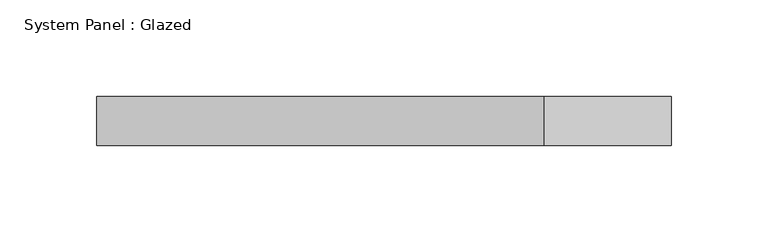
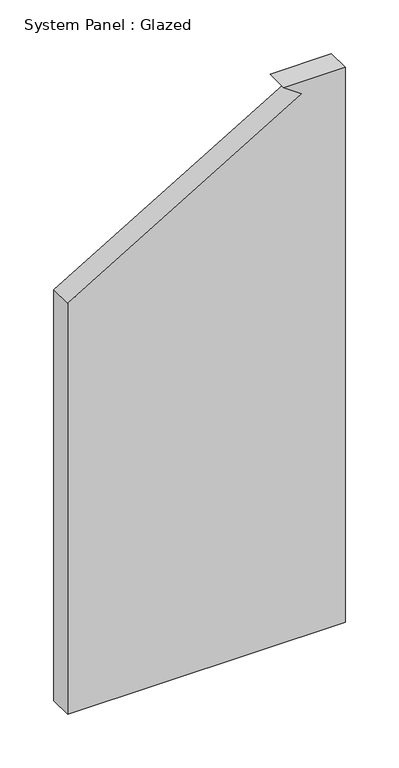
"""IFC4 building model written with IfcOpenShell, lengths in millimetres: plate geometry, System Panel : Glazed."""

from ifc_helpers import new_model, si_unit, frame, origin, place, context, project, spatial, polyline, outline, extrude, source, transform, mapped, element, save


def system_panel_glazed_2554e476(model_context):
    return source(origin(), model_context, "Body", "SweptSolid", [
        extrude(outline(polyline([(0.0, -148.7667393), (0.0, 148.7667393), (628.65, 148.7667393), (628.65, 83.0508137), (614.9480806, 102.5167269), (465.5992108, -148.7667393), (0.0, -148.7667393)])), frame((0.0, 19.05, 0.0), z_axis=(0.0, 1.0, 0.0), x_axis=(0.0, 0.0, 1.0)), (0.0, 0.0, 1.0), 25.4),
    ])


if __name__ == "__main__":
    model = new_model("IFC4")
    model_context = context("Model", 3, world=origin())
    ifc_project = project(units=[si_unit("LENGTHUNIT", "METRE", prefix="MILLI")], contexts=[model_context])
    site = spatial("IfcSite", under=ifc_project)
    building = spatial("IfcBuilding", under=site)
    placement = place(None, origin())
    system_panel_glazed_shape = system_panel_glazed_2554e476(model_context)
    element("IfcPlate", 1, ObjectType="System Panel : Glazed", at=placement, inside=building, context=model_context, shape_type="MappedRepresentation", body=[
        mapped(system_panel_glazed_shape, transform((0.0, 0.0, 0.0), x_axis=(1.0, 0.0, 0.0), y_axis=(0.0, 1.0, 0.0), z_axis=(0.0, 0.0, 1.0))),
    ])
    save(model, "model.ifc")

# Revit data of these elements
# Type "System Panel : Glazed"
#   Construction Type Id = "GSP4R"
#   Analytic Construction = "1/8 in Pilkington single glazing"
#   Visual Light Transmittance = 0.9
#   Solar Heat Gain Coefficient = 0.86
#   Heat Transfer Coefficient (U) = 1.18115 BTU/(h·ft²·°F)
#   Define Thermal Properties by = 1
# Element 1 (IfcPlate, "System Panel : Glazed")
#   Materials on its faces: "Glass"
# Materials
#   "Glass": class "Glass", colour RGB 0 128 192, transparency 0.75, Description = "Soda Lime Glass", Cost = 0
